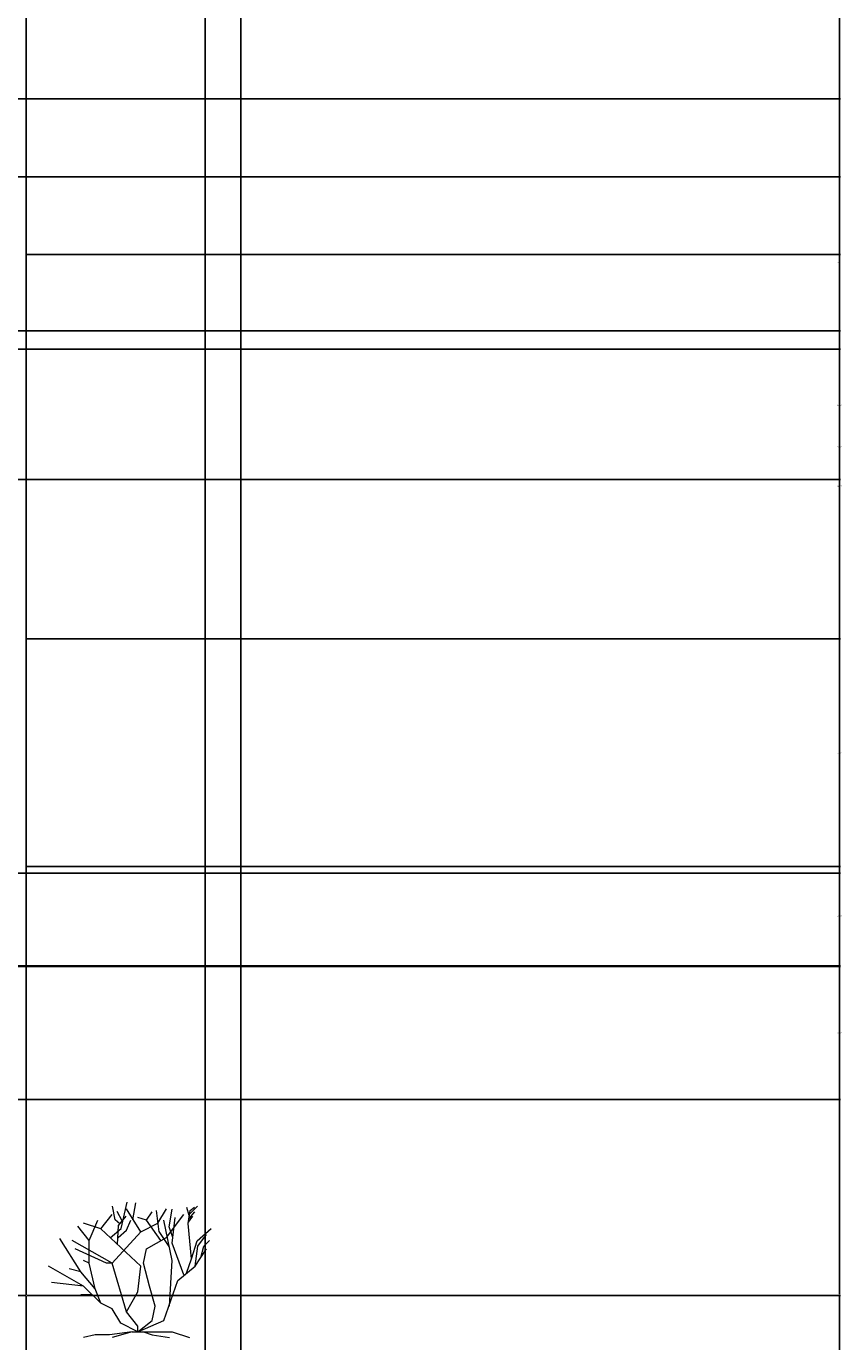
# Model space of a CAD drawing. Units: inches. Extents: x -47 to 496, y -43 to 706.
# Tile 4 of 6: x 359 to 496, y 123 to 344. Entities that reach past the tile are written whole.
import ezdxf

# ---------------------------------------------------------------- set-up
doc = ezdxf.new("R2010")
doc.units = ezdxf.units.IN
for name, color, linetype, lineweight in [('A-ANNO-DIMS', 2, 'Continuous', 18), ('C-PROP', 7, 'Continuous', 25), ('L-PLNT', 3, 'Continuous', 13)]:
    doc.layers.add(name, color=color, linetype=linetype, lineweight=lineweight)
doc.styles.get("Standard").update_dxf_attribs({"font": 'arial.ttf'})
doc.dimstyles.get("Standard").update_dxf_attribs({"dimtxt": 0.18, "dimasz": 0.18, "dimexe": 0.18, "dimexo": 0.0625, "dimgap": 0.09, "dimtad": 0, "dimtih": 1, "dimtoh": 1, "dimdec": 4, "dimzin": 0, "dimdsep": 46, "dimtxsty": 'Standard', "dimcen": 0.09, "dimadec": 0, "dimazin": 0, "dimtfac": 1, "dimtdec": 4, "dimtofl": 0, "dimtmove": 0, "dimatfit": 3, "dimfxl": 1, "dimtolj": 1, "dimtzin": 0, "dimarcsym": 0})

# ---------------------------------------------------------------- blocks, each defined once
blk = doc.blocks.new('*U6')
for p, q in [((-11.433, 18.289), (-10.457, 22.749)), ((-9.48, 19.775), (-8.992, 22.592)), ((-14.88, 18.24), (-12.96, 20.64)), ((-12.471, 19.775), (-12.898, 22.044)), ((-11.28, 19.619), (-12.104, 21.184)), ((-11.921, 18.836), (-10.64, 20.401)), ((-8.16, 17.76), (-10.56, 21.6)), ((-7.2, 19.68), (-8.64, 20.16)), ((-7.2, 19.68), (-6.24, 21.12)), ((-5.086, 17.741), (-5.513, 21.34)), ((-5.28, 19.2), (-3.84, 21.6)), ((-3.84, 16.8), (-0.96, 20.64)), ((-3.377, 18.602), (-2.888, 21.575)), ((-2.88, 15.84), (-2.4, 20.16)), ((-0.508, 21.888), (-0.081, 20.558)), ((-0.203, 19.149), (0.102, 21.34)), ((-0.142, 19.384), (0.59, 20.401)), ((-0.02, 20.01), (0.896, 21.105)), ((0.041, 20.714), (1.384, 22.044)), ((0.102, 21.34), (0.835, 21.888)), ((-16.8, 16.32), (-18.72, 18.72)), ((-14.88, 18.24), (-17.76, 19.2)), ((-16.8, 16.32), (-15.36, 19.68)), ((-8.16, 12), (-14.88, 18.24)), ((-13.325, 16.724), (-11.433, 18.289)), ((-12.96, 12.48), (-8.16, 17.76)), ((-11.677, 19.071), (-12.471, 19.775)), ((-12.043, 15.628), (-11.921, 18.836)), ((-11.982, 16.802), (-10.579, 18.054)), ((-10.579, 18.054), (-9.846, 19.697)), ((-8.16, 17.76), (-5.28, 19.2)), ((-4.8, 16.32), (-7.2, 19.68)), ((-3.377, 15.315), (-5.086, 17.819)), ((-2.88, 12.96), (-4.32, 19.68)), ((-2.766, 16.802), (-3.377, 18.602)), ((0.346, 13.203), (-0.203, 19.149)), ((1.323, 16.254), (3.642, 18.289)), ((-18.24, 11.04), (-21.755, 16.655)), ((-12.96, 12.48), (-19.68, 16.32)), ((-16.8, 12.48), (-16.8, 16.32)), ((-7.2, 14.88), (-3.84, 16.8)), ((-0.96, 10.56), (-2.88, 15.84)), ((0.346, 13.203), (1.323, 16.254)), ((1.44, 15.36), (2.88, 17.28)), ((2.4, 15.36), (3.36, 16.32)), ((-13.92, 12.48), (-19.2, 14.88)), ((-7.68, 12.48), (-7.2, 14.88)), ((0.96, 12), (1.44, 15.36)), ((0.96, 12), (2.88, 14.88)), ((1.92, 13.44), (2.4, 15.36)), ((-17.76, 8.64), (-23.663, 11.961)), ((-18.24, 11.04), (-20.16, 11.52)), ((-15.84, 8.16), (-18.24, 11.04)), ((-16.8, 12.48), (-17.76, 12.96)), ((-15.84, 8.16), (-16.8, 12.48)), ((-12.96, 12.48), (-13.92, 12.48)), ((-10.56, 4.32), (-12.96, 12.48)), ((-8.64, 7.68), (-8.16, 12)), ((-6.72, 8.64), (-7.68, 12.48)), ((-3.36, 5.28), (-2.88, 12.96)), ((-1.92, 9.6), (0.96, 12)), ((-0.48, 10.8), (0.346, 13.203)), ((-17.76, 8.64), (-23.128, 9.222)), ((-4.32, 2.88), (-1.92, 9.6)), ((-16.32, 7.2), (-18.24, 7.2)), ((-14.88, 5.76), (-17.76, 8.64)), ((-14.88, 5.76), (-15.84, 8.16)), ((-10.56, 4.32), (-8.64, 7.68)), ((-5.76, 5.28), (-6.72, 8.64)), ((-12.96, 4.8), (-14.88, 5.76)), ((-11.52, 2.4), (-12.96, 4.8)), ((-6.24, 2.88), (-5.76, 5.28)), ((-8.64, 0.96), (-11.52, 2.4)), ((-8.64, 1.92), (-10.56, 4.32)), ((-8.64, 0.96), (-4.32, 2.88)), ((-8.64, 0.96), (-6.24, 2.88)), ((-15.84, 0.48), (-17.76, 0)), ((-13.44, 0.48), (-15.84, 0.48)), ((-9.6, 0.96), (-13.44, 0.48)), ((-9.6, 0.96), (-12.96, 0)), ((-9.6, 0.96), (-7.68, 0.96)), ((-8.64, 0.96), (-8.64, 1.92)), ((-8.64, 0.96), (-2.88, 0.96)), ((-7.68, 0.96), (-6.24, 0.48)), ((-6.24, 0.48), (-3.36, 0)), ((-2.88, 0.96), (0, 0))]:
    blk.add_line(p, q)
blk = doc.blocks.new('*D18')
at = {"layer": 'A-ANNO-DIMS', "color": 0, "lineweight": -2, "transparency": 16777216}
for p, q in [((359.52, 635.47), (496.14, 635.47)), ((495.96, 635.29), (495.96, 419.4)), ((495.96, 203.15), (495.96, 419.04)), ((359.52, 202.97), (496.14, 202.97))]:
    blk.add_line(p, q, dxfattribs=at)
at = {"layer": 'A-ANNO-DIMS', "color": 0, "transparency": 16777216}
for points in [[(495.93, 635.29), (495.99, 635.29), (495.96, 635.47)], [(495.93, 203.15), (495.99, 203.15), (495.96, 202.97)]]:
    blk.add_solid(points, dxfattribs=at)
at = {"layer": 'Defpoints', "color": 0, "transparency": 16777216}
for p in [(359.45, 635.47), (495.96, 635.47), (359.45, 202.97)]:
    blk.add_point(p, dxfattribs=at)
at = {"layer": 'A-ANNO-DIMS', "color": 0, "transparency": 16777216, "insert": (495.96, 419.22), "char_height": 0.18, "attachment_point": 5}
blk.add_mtext('\\A1;432.5', dxfattribs=at)
blk = doc.blocks.new('*D19')
at = {"layer": 'A-ANNO-DIMS', "color": 0, "lineweight": -2, "transparency": 16777216}
for p, q in [((359.52, 202.97), (496.14, 202.97)), ((495.96, 202.79), (495.96, 167.15)), ((495.96, 131.15), (495.96, 166.79)), ((359.52, 130.97), (496.14, 130.97))]:
    blk.add_line(p, q, dxfattribs=at)
at = {"layer": 'A-ANNO-DIMS', "color": 0, "transparency": 16777216}
for points in [[(495.93, 202.79), (495.99, 202.79), (495.96, 202.97)], [(495.93, 131.15), (495.99, 131.15), (495.96, 130.97)]]:
    blk.add_solid(points, dxfattribs=at)
at = {"layer": 'Defpoints', "color": 0, "transparency": 16777216}
for p in [(359.45, 202.97), (495.96, 202.97), (359.45, 130.97)]:
    blk.add_point(p, dxfattribs=at)
at = {"layer": 'A-ANNO-DIMS', "color": 0, "transparency": 16777216, "insert": (495.96, 166.97), "char_height": 0.18, "attachment_point": 5}
blk.add_mtext('\\A1;72', dxfattribs=at)
blk = doc.blocks.new('*D20')
at = {"layer": 'A-ANNO-DIMS', "color": 0, "lineweight": -2, "transparency": 16777216}
for p, q in [((359.52, 130.97), (496.14, 130.97)), ((495.96, 130.79), (495.96, 92.15)), ((495.96, 53.15), (495.96, 91.79)), ((395.52, 52.97), (496.14, 52.97))]:
    blk.add_line(p, q, dxfattribs=at)
at = {"layer": 'A-ANNO-DIMS', "color": 0, "transparency": 16777216}
for points in [[(495.93, 130.79), (495.99, 130.79), (495.96, 130.97)], [(495.93, 53.15), (495.99, 53.15), (495.96, 52.97)]]:
    blk.add_solid(points, dxfattribs=at)
at = {"layer": 'Defpoints', "color": 0, "transparency": 16777216}
for p in [(359.45, 130.97), (495.96, 130.97), (395.45, 52.97)]:
    blk.add_point(p, dxfattribs=at)
at = {"layer": 'A-ANNO-DIMS', "color": 0, "transparency": 16777216, "insert": (495.96, 91.97), "char_height": 0.18, "attachment_point": 5}
blk.add_mtext('\\A1;78', dxfattribs=at)
blk = doc.blocks.new('*D21')
at = {"layer": 'A-ANNO-DIMS', "color": 0, "lineweight": -2, "transparency": 16777216}
for p, q in [((213.95, 130.91), (213.95, -42.84)), ((359.45, 130.91), (359.45, -42.84)), ((214.13, -42.66), (286.32, -42.66)), ((359.27, -42.66), (287.09, -42.66))]:
    blk.add_line(p, q, dxfattribs=at)
at = {"layer": 'A-ANNO-DIMS', "color": 0, "transparency": 16777216}
for points in [[(214.13, -42.63), (214.13, -42.69), (213.95, -42.66)], [(359.27, -42.63), (359.27, -42.69), (359.45, -42.66)]]:
    blk.add_solid(points, dxfattribs=at)
at = {"layer": 'Defpoints', "color": 0, "transparency": 16777216}
for p in [(213.95, 130.97), (359.45, 130.97), (359.45, -42.66)]:
    blk.add_point(p, dxfattribs=at)
at = {"layer": 'A-ANNO-DIMS', "color": 0, "transparency": 16777216, "insert": (286.7, -42.66), "char_height": 0.18, "attachment_point": 5}
blk.add_mtext('\\A1;145.5', dxfattribs=at)
blk = doc.blocks.new('*D23')
at = {"layer": 'A-ANNO-DIMS', "color": 0, "lineweight": -2, "transparency": 16777216}
for p, q in [((262.58, 186.29), (496.14, 186.29)), ((495.96, 186.11), (495.96, 175.24)), ((495.96, 164.01), (495.96, 174.88)), ((262.58, 163.83), (496.14, 163.83))]:
    blk.add_line(p, q, dxfattribs=at)
at = {"layer": 'A-ANNO-DIMS', "color": 0, "transparency": 16777216}
for points in [[(495.93, 186.11), (495.99, 186.11), (495.96, 186.29)], [(495.93, 164.01), (495.99, 164.01), (495.96, 163.83)]]:
    blk.add_solid(points, dxfattribs=at)
at = {"layer": 'Defpoints', "color": 0, "transparency": 16777216}
for p in [(262.51, 186.29), (495.96, 186.29), (262.51, 163.83)]:
    blk.add_point(p, dxfattribs=at)
at = {"layer": 'A-ANNO-DIMS', "color": 0, "transparency": 16777216, "insert": (495.96, 175.06), "char_height": 0.18, "attachment_point": 5}
blk.add_mtext('\\A1;22.45', dxfattribs=at)
blk = doc.blocks.new('*D28')
at = {"layer": 'A-ANNO-DIMS', "color": 0, "lineweight": -2, "transparency": 16777216}
for p, q in [((346.5, 165.93), (346.5, 705.7)), ((346.68, 705.52), (352.52, 705.52)), ((359.27, 705.52), (353.43, 705.52)), ((359.45, 131.03), (359.45, 705.7))]:
    blk.add_line(p, q, dxfattribs=at)
at = {"layer": 'A-ANNO-DIMS', "color": 0, "transparency": 16777216}
for points in [[(346.68, 705.55), (346.68, 705.49), (346.5, 705.52)], [(359.27, 705.55), (359.27, 705.49), (359.45, 705.52)]]:
    blk.add_solid(points, dxfattribs=at)
at = {"layer": 'Defpoints', "color": 0, "transparency": 16777216}
for p in [(359.45, 705.52), (346.5, 165.87), (359.45, 130.97)]:
    blk.add_point(p, dxfattribs=at)
at = {"layer": 'A-ANNO-DIMS', "color": 0, "transparency": 16777216, "insert": (352.98, 705.52), "char_height": 0.18, "attachment_point": 5}
blk.add_mtext('\\A1;12.954', dxfattribs=at)
blk = doc.blocks.new('*D29')
at = {"layer": 'A-ANNO-DIMS', "color": 0, "lineweight": -2, "transparency": 16777216}
for p, q in [((359.52, 202.97), (496.14, 202.97)), ((495.96, 202.79), (495.96, 194.76)), ((495.96, 186.36), (495.96, 194.4)), ((346.56, 186.18), (496.14, 186.18))]:
    blk.add_line(p, q, dxfattribs=at)
at = {"layer": 'A-ANNO-DIMS', "color": 0, "transparency": 16777216}
for points in [[(495.93, 202.79), (495.99, 202.79), (495.96, 202.97)], [(495.93, 186.36), (495.99, 186.36), (495.96, 186.18)]]:
    blk.add_solid(points, dxfattribs=at)
at = {"layer": 'Defpoints', "color": 0, "transparency": 16777216}
for p in [(359.45, 202.97), (495.96, 202.97), (346.5, 186.18)]:
    blk.add_point(p, dxfattribs=at)
at = {"layer": 'A-ANNO-DIMS', "color": 0, "transparency": 16777216, "insert": (495.96, 194.58), "char_height": 0.18, "attachment_point": 5}
blk.add_mtext('\\A1;16.787', dxfattribs=at)
blk = doc.blocks.new('*D31')
at = {"layer": 'A-ANNO-DIMS', "color": 0, "lineweight": -2, "transparency": 16777216}
for p, q in [((285.55, 151.67), (-47.29, 151.67)), ((-47.11, 151.49), (-47.11, 141.5)), ((-47.11, 131.15), (-47.11, 141.14)), ((359.39, 130.97), (-47.29, 130.97))]:
    blk.add_line(p, q, dxfattribs=at)
at = {"layer": 'A-ANNO-DIMS', "color": 0, "transparency": 16777216}
for points in [[(-47.14, 151.49), (-47.08, 151.49), (-47.11, 151.67)], [(-47.14, 131.15), (-47.08, 131.15), (-47.11, 130.97)]]:
    blk.add_solid(points, dxfattribs=at)
at = {"layer": 'Defpoints', "color": 0, "transparency": 16777216}
for p in [(285.61, 151.67), (-47.11, 130.97), (359.45, 130.97)]:
    blk.add_point(p, dxfattribs=at)
at = {"layer": 'A-ANNO-DIMS', "color": 0, "transparency": 16777216, "insert": (-47.11, 141.32), "char_height": 0.18, "attachment_point": 5}
blk.add_mtext('\\A1;20.695', dxfattribs=at)
blk = doc.blocks.new('*D76')
at = {"layer": 'A-ANNO-DIMS', "color": 0, "lineweight": -2, "transparency": 16777216}
for p, q in [((359.52, 241.14), (496.14, 241.14)), ((495.96, 240.96), (495.96, 222.24)), ((495.96, 203.15), (495.96, 221.87)), ((359.52, 202.97), (496.14, 202.97))]:
    blk.add_line(p, q, dxfattribs=at)
at = {"layer": 'A-ANNO-DIMS', "color": 0, "transparency": 16777216}
for points in [[(495.93, 240.96), (495.99, 240.96), (495.96, 241.14)], [(495.93, 203.15), (495.99, 203.15), (495.96, 202.97)]]:
    blk.add_solid(points, dxfattribs=at)
at = {"layer": 'Defpoints', "color": 0, "transparency": 16777216}
for p in [(359.45, 241.14), (495.96, 241.14), (359.45, 202.97)]:
    blk.add_point(p, dxfattribs=at)
at = {"layer": 'A-ANNO-DIMS', "color": 0, "transparency": 16777216, "insert": (495.96, 222.05), "char_height": 0.18, "attachment_point": 5}
blk.add_mtext('\\A1;38.17', dxfattribs=at)
blk = doc.blocks.new('*D77')
at = {"layer": 'A-ANNO-DIMS', "color": 0, "lineweight": -2, "transparency": 16777216}
for p, q in [((359.52, 305.68), (496.14, 305.68)), ((495.96, 305.5), (495.96, 273.59)), ((495.96, 241.32), (495.96, 273.23)), ((359.52, 241.14), (496.14, 241.14))]:
    blk.add_line(p, q, dxfattribs=at)
at = {"layer": 'A-ANNO-DIMS', "color": 0, "transparency": 16777216}
for points in [[(495.93, 305.5), (495.99, 305.5), (495.96, 305.68)], [(495.93, 241.32), (495.99, 241.32), (495.96, 241.14)]]:
    blk.add_solid(points, dxfattribs=at)
at = {"layer": 'Defpoints', "color": 0, "transparency": 16777216}
for p in [(359.45, 305.68), (495.96, 305.68), (359.45, 241.14)]:
    blk.add_point(p, dxfattribs=at)
at = {"layer": 'A-ANNO-DIMS', "color": 0, "transparency": 16777216, "insert": (495.96, 273.41), "char_height": 0.18, "attachment_point": 5}
blk.add_mtext('\\A1;64.55', dxfattribs=at)
blk = doc.blocks.new('*D80')
at = {"layer": 'A-ANNO-DIMS', "color": 0, "lineweight": -2, "transparency": 16777216}
for p, q in [((218.52, 292.83), (496.14, 292.83)), ((495.96, 292.65), (495.96, 280.53)), ((495.96, 268.06), (495.96, 280.17)), ((218.52, 267.88), (496.14, 267.88))]:
    blk.add_line(p, q, dxfattribs=at)
at = {"layer": 'A-ANNO-DIMS', "color": 0, "transparency": 16777216}
for points in [[(495.93, 292.65), (495.99, 292.65), (495.96, 292.83)], [(495.93, 268.06), (495.99, 268.06), (495.96, 267.88)]]:
    blk.add_solid(points, dxfattribs=at)
at = {"layer": 'Defpoints', "color": 0, "transparency": 16777216}
for p in [(218.45, 292.83), (495.96, 292.83), (218.45, 267.88)]:
    blk.add_point(p, dxfattribs=at)
at = {"layer": 'A-ANNO-DIMS', "color": 0, "transparency": 16777216, "insert": (495.96, 280.35), "char_height": 0.18, "attachment_point": 5}
blk.add_mtext('\\A1;24.946', dxfattribs=at)
blk = doc.blocks.new('*D82')
at = {"layer": 'A-ANNO-DIMS', "color": 0, "lineweight": -2, "transparency": 16777216}
for p, q in [((108.88, 331.8), (496.14, 331.8)), ((495.96, 331.62), (495.96, 267)), ((495.96, 202.02), (495.96, 266.64)), ((131.48, 201.84), (496.14, 201.84))]:
    blk.add_line(p, q, dxfattribs=at)
at = {"layer": 'A-ANNO-DIMS', "color": 0, "transparency": 16777216}
for points in [[(495.93, 331.62), (495.99, 331.62), (495.96, 331.8)], [(495.93, 202.02), (495.99, 202.02), (495.96, 201.84)]]:
    blk.add_solid(points, dxfattribs=at)
at = {"layer": 'Defpoints', "color": 0, "transparency": 16777216}
for p in [(108.82, 331.8), (131.41, 201.84), (495.96, 201.84)]:
    blk.add_point(p, dxfattribs=at)
at = {"layer": 'A-ANNO-DIMS', "color": 0, "transparency": 16777216, "insert": (495.96, 266.82), "char_height": 0.18, "attachment_point": 5}
blk.add_mtext('\\A1;129.95', dxfattribs=at)
blk = doc.blocks.new('*D87')
at = {"layer": 'A-ANNO-DIMS', "color": 0, "lineweight": -2, "transparency": 16777216}
for p, q in [((308.33, 318.72), (496.14, 318.72)), ((495.96, 318.54), (495.96, 304.44)), ((495.96, 289.97), (495.96, 304.07)), ((308.33, 289.79), (496.14, 289.79))]:
    blk.add_line(p, q, dxfattribs=at)
at = {"layer": 'A-ANNO-DIMS', "color": 0, "transparency": 16777216}
for points in [[(495.93, 318.54), (495.99, 318.54), (495.96, 318.72)], [(495.93, 289.97), (495.99, 289.97), (495.96, 289.79)]]:
    blk.add_solid(points, dxfattribs=at)
at = {"layer": 'Defpoints', "color": 0, "transparency": 16777216}
for p in [(308.27, 318.72), (495.96, 318.72), (308.27, 289.79)]:
    blk.add_point(p, dxfattribs=at)
at = {"layer": 'A-ANNO-DIMS', "color": 0, "transparency": 16777216, "insert": (495.96, 304.26), "char_height": 0.18, "attachment_point": 5}
blk.add_mtext('\\A1;28.94', dxfattribs=at)

msp = doc.modelspace()

# ---------------------------------------------------------------- linework, layer by layer
at = {"layer": 'C-PROP'}
for p, q in [((395.4545, 671.4711), (395.4545, 52.9711)), ((389.4545, 665.4711), (389.4545, 58.9711))]:
    msp.add_line(p, q, dxfattribs=at)

# ---------------------------------------------------------------- block references
at = {"layer": 'L-PLNT'}
msp.add_blockref('*U6', (386.8339, 123.8798), dxfattribs=at)

# ---------------------------------------------------------------- dimensions: what is measured, and where the dimension line sits
at = {"layer": 'A-ANNO-DIMS'}
for base, p1, p2, override, picture, middle in [((359.45448, 705.52106), (346.5, 165.86638), (359.45448, 130.97106), {"dimdec": 3, "dimlfac": 1, "dimrnd": 0, "dimzin": 0, "dimdsep": 46, "dimlunit": 2}, '*D28', (352.97724, 705.52106)), ((359.4545, -42.6632), (213.9545, 130.9711), (359.4545, 130.9711), {"dimdec": 1, "dimlfac": 1, "dimrnd": 0, "dimzin": 0, "dimdsep": 46, "dimlunit": 2}, '*D21', (286.7045, -42.6632))]:
    dim = msp.add_linear_dim(base=base, p1=p1, p2=p2, dimstyle='Standard', override=override, dxfattribs=at)
    dim.commit()
    dim.dimension.update_dxf_attribs({"geometry": picture, "text_midpoint": middle})
for base, p1, p2, override, picture, middle in [((495.9572, 635.4711), (359.4545, 202.9711), (359.4545, 635.4711), {"dimdec": 1, "dimlfac": 1, "dimrnd": 0, "dimzin": 0, "dimdsep": 46, "dimlunit": 2}, '*D18', (495.9572, 419.2211)), ((495.9572, 201.8438), (108.8164, 331.7986), (131.4128, 201.8438), {"dimdec": 2, "dimlfac": 1, "dimrnd": 0, "dimzin": 0, "dimdsep": 46, "dimlunit": 2}, '*D82', (495.9572, 266.8212)), ((495.9572, 318.7246), (308.2664, 289.7875), (308.2664, 318.7246), {"dimdec": 2, "dimlfac": 1, "dimrnd": 0, "dimzin": 0, "dimdsep": 46, "dimlunit": 2}, '*D87', (495.9572, 304.2561)), ((495.9572, 305.6843), (359.4545, 241.1376), (359.4545, 305.6843), {"dimdec": 2, "dimlfac": 1, "dimrnd": 0, "dimzin": 0, "dimdsep": 46, "dimlunit": 2}, '*D77', (495.9572, 273.4109)), ((495.9572, 292.8257), (218.4545, 267.8798), (218.4545, 292.8257), {"dimdec": 3, "dimlfac": 1, "dimrnd": 0, "dimzin": 0, "dimdsep": 46, "dimlunit": 2}, '*D80', (495.9572, 280.3528)), ((495.9572, 241.1376), (359.4545, 202.9711), (359.4545, 241.1376), {"dimdec": 2, "dimlfac": 1, "dimrnd": 0, "dimzin": 0, "dimdsep": 46, "dimlunit": 2}, '*D76', (495.9572, 222.0543)), ((495.9572, 202.9711), (346.5, 186.184), (359.4545, 202.9711), {"dimdec": 3, "dimlfac": 1, "dimrnd": 0, "dimzin": 0, "dimdsep": 46, "dimlunit": 2}, '*D29', (495.9572, 194.5775)), ((495.9572, 202.9711), (359.4545, 130.9711), (359.4545, 202.9711), {"dimdec": 0, "dimlfac": 1, "dimrnd": 0, "dimzin": 0, "dimdsep": 46, "dimlunit": 2}, '*D19', (495.9572, 166.9711)), ((495.9572, 186.2855), (262.5138, 163.8346), (262.5138, 186.2855), {"dimdec": 2, "dimlfac": 1, "dimrnd": 0, "dimzin": 0, "dimdsep": 46, "dimlunit": 2}, '*D23', (495.9572, 175.0601)), ((-47.1058, 130.9711), (285.6085, 151.6661), (359.4545, 130.9711), {"dimdec": 3, "dimlfac": 1, "dimrnd": 0, "dimzin": 0, "dimdsep": 46, "dimlunit": 2}, '*D31', (-47.1058, 141.3186)), ((495.9572, 130.9711), (395.4545, 52.9711), (359.4545, 130.9711), {"dimdec": 0, "dimlfac": 1, "dimrnd": 0, "dimzin": 0, "dimdsep": 46, "dimlunit": 2}, '*D20', (495.9572, 91.9711))]:
    dim = msp.add_linear_dim(base=base, p1=p1, p2=p2, angle=90, dimstyle='Standard', override=override, dxfattribs=at)
    dim.commit()
    dim.dimension.update_dxf_attribs({"geometry": picture, "text_midpoint": middle})

doc.saveas('drawing.dxf')
